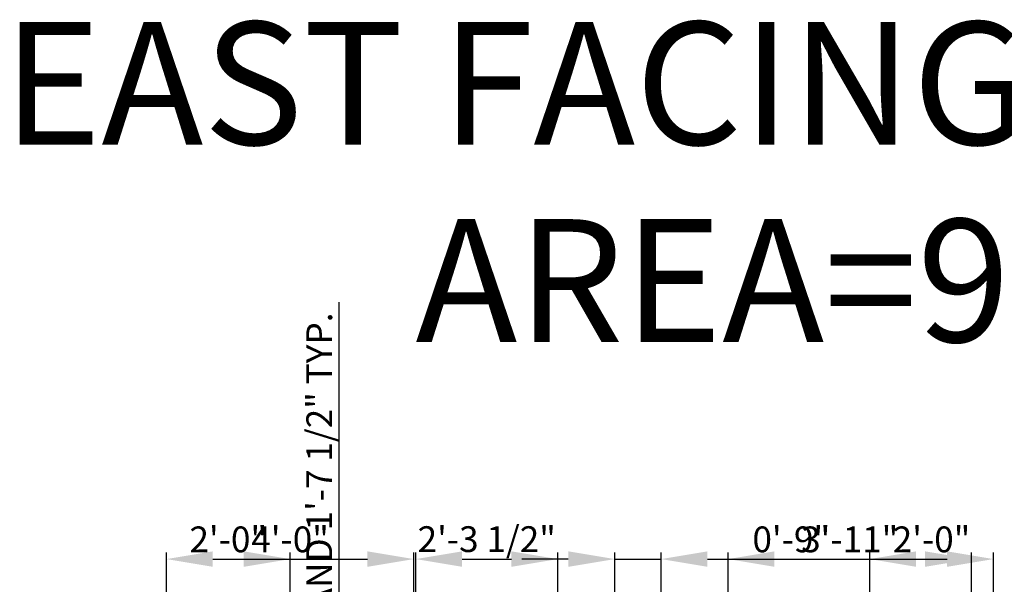
# Model space of a CAD drawing. Units: inches. Extents: x 2265 to 2807, y 1544 to 2401.
# Tile 6 of 9: x 2340 to 2531, y 2291 to 2401. Entities that reach past the tile are written whole.
import ezdxf

# ---------------------------------------------------------------- set-up
doc = ezdxf.new("R2010")
doc.units = ezdxf.units.IN
doc.layers.add('A-ANNO-DIMS', color=2, linetype='Continuous', lineweight=18)
doc.layers.add('A-ANNO-TITL', color=7, linetype='Continuous', lineweight=35)
doc.styles.get("Standard").update_dxf_attribs({"font": 'arial.ttf', "height": 5})
doc.dimstyles.new('ISO-25', dxfattribs={"dimtxt": 5, "dimasz": 9, "dimexe": 1.25, "dimexo": 0.625, "dimtad": 1, "dimlunit": 3, "dimtxsty": 'Standard', "dimcen": 2.5, "dimadec": 0, "dimazin": 0, "dimtfac": 1, "dimtmove": 0, "dimatfit": 3, "dimfxl": 1, "dimarcsym": 0})

# ---------------------------------------------------------------- blocks, each defined once
blk = doc.blocks.new('*D31')
at = {"layer": 'A-ANNO-DIMS', "color": 0, "lineweight": -2, "transparency": 16777216}
for p, q in [((2401.62, 2246.73), (2401.62, 2346.21)), ((2399.29, 2246.73), (2402.87, 2246.73)), ((2401.62, 2236.05), (2401.62, 2237.73)), ((2399.29, 2227.05), (2402.87, 2227.05))]:
    blk.add_line(p, q, dxfattribs=at)
at = {"layer": 'A-ANNO-DIMS', "color": 0, "lineweight": 100, "transparency": 16777216}
for points in [[(2400.12, 2237.73), (2403.12, 2237.73), (2401.62, 2246.73)], [(2400.12, 2236.05), (2403.12, 2236.05), (2401.62, 2227.05)]]:
    blk.add_solid(points, dxfattribs=at)
at = {"layer": 'Defpoints', "color": 0, "lineweight": 100, "transparency": 16777216}
for p in [(2398.67, 2246.73), (2401.62, 2246.73), (2398.67, 2227.05)]:
    blk.add_point(p, dxfattribs=at)
at = {"layer": 'A-ANNO-DIMS', "color": 0, "transparency": 16777216, "insert": (2398.41, 2300.97), "char_height": 5, "attachment_point": 5, "rotation": 90}
blk.add_mtext('NIGHTSTAND 1\'-7 1/2" TYP.', dxfattribs=at)
blk = doc.blocks.new('*D40')
at = {"layer": 'A-ANNO-DIMS', "color": 0, "lineweight": -2, "transparency": 16777216}
for p, q in [((2368.1, 2005.86), (2368.1, 2297.59)), ((2392.1, 2005.86), (2392.1, 2297.59)), ((2377.1, 2296.34), (2383.1, 2296.34))]:
    blk.add_line(p, q, dxfattribs=at)
at = {"layer": 'A-ANNO-DIMS', "color": 0, "lineweight": 100, "transparency": 16777216}
for points in [[(2377.1, 2297.84), (2377.1, 2294.84), (2368.1, 2296.34)], [(2383.1, 2297.84), (2383.1, 2294.84), (2392.1, 2296.34)]]:
    blk.add_solid(points, dxfattribs=at)
at = {"layer": 'Defpoints', "color": 0, "lineweight": 100, "transparency": 16777216}
for p in [(2392.1, 2296.34), (2368.1, 2005.23), (2392.1, 2005.23)]:
    blk.add_point(p, dxfattribs=at)
at = {"layer": 'A-ANNO-DIMS', "color": 0, "transparency": 16777216, "insert": (2380.1, 2299.52), "char_height": 5, "attachment_point": 5}
blk.add_mtext('2\'-0"', dxfattribs=at)
blk = doc.blocks.new('*D43')
at = {"layer": 'A-ANNO-DIMS', "color": 0, "lineweight": -2, "transparency": 16777216}
for p, q in [((2416.49, 1959.08), (2416.49, 2297.59)), ((2444.05, 1959.08), (2444.05, 2297.59)), ((2425.49, 2296.34), (2435.05, 2296.34))]:
    blk.add_line(p, q, dxfattribs=at)
at = {"layer": 'A-ANNO-DIMS', "color": 0, "lineweight": 100, "transparency": 16777216}
for points in [[(2425.49, 2297.84), (2425.49, 2294.84), (2416.49, 2296.34)], [(2435.05, 2297.84), (2435.05, 2294.84), (2444.05, 2296.34)]]:
    blk.add_solid(points, dxfattribs=at)
at = {"layer": 'Defpoints', "color": 0, "lineweight": 100, "transparency": 16777216}
for p in [(2444.05, 2296.34), (2416.49, 1958.45), (2444.05, 1958.45)]:
    blk.add_point(p, dxfattribs=at)
at = {"layer": 'A-ANNO-DIMS', "color": 0, "transparency": 16777216, "insert": (2430.27, 2299.56), "char_height": 5, "attachment_point": 5}
blk.add_mtext('2\'-3 1/2"', dxfattribs=at)
blk = doc.blocks.new('*D47')
at = {"layer": 'A-ANNO-DIMS', "color": 0, "lineweight": -2, "transparency": 16777216}
for p, q in [((2455.1, 2124.36), (2455.1, 2297.59)), ((2464.1, 2124.36), (2464.1, 2297.59)), ((2446.1, 2296.34), (2437.1, 2296.34)), ((2455.1, 2296.34), (2464.1, 2296.34)), ((2473.1, 2296.34), (2496.64, 2296.34))]:
    blk.add_line(p, q, dxfattribs=at)
at = {"layer": 'A-ANNO-DIMS', "color": 0, "lineweight": 100, "transparency": 16777216}
for points in [[(2446.1, 2297.84), (2446.1, 2294.84), (2455.1, 2296.34)], [(2473.1, 2297.84), (2473.1, 2294.84), (2464.1, 2296.34)]]:
    blk.add_solid(points, dxfattribs=at)
at = {"layer": 'Defpoints', "color": 0, "lineweight": 100, "transparency": 16777216}
for p in [(2464.1, 2296.34), (2455.1, 2123.73), (2464.1, 2123.73)]:
    blk.add_point(p, dxfattribs=at)
at = {"layer": 'A-ANNO-DIMS', "color": 0, "transparency": 16777216, "insert": (2489.37, 2299.52), "char_height": 5, "attachment_point": 5}
blk.add_mtext('0\'-9"', dxfattribs=at)
blk = doc.blocks.new('*D54')
at = {"layer": 'A-ANNO-DIMS', "color": 0, "lineweight": -2, "transparency": 16777216}
for p, q in [((2368.1, 2247.36), (2368.1, 2297.59)), ((2416.1, 2247.36), (2416.1, 2297.59)), ((2377.1, 2296.34), (2407.1, 2296.34))]:
    blk.add_line(p, q, dxfattribs=at)
at = {"layer": 'A-ANNO-DIMS', "color": 0, "lineweight": 100, "transparency": 16777216}
for points in [[(2377.1, 2297.84), (2377.1, 2294.84), (2368.1, 2296.34)], [(2407.1, 2297.84), (2407.1, 2294.84), (2416.1, 2296.34)]]:
    blk.add_solid(points, dxfattribs=at)
at = {"layer": 'Defpoints', "color": 0, "lineweight": 100, "transparency": 16777216}
for p in [(2416.1, 2296.34), (2368.1, 2246.73), (2416.1, 2246.73)]:
    blk.add_point(p, dxfattribs=at)
at = {"layer": 'A-ANNO-DIMS', "color": 0, "transparency": 16777216, "insert": (2392.1, 2299.52), "char_height": 5, "attachment_point": 5}
blk.add_mtext('4\'-0"', dxfattribs=at)
blk = doc.blocks.new('*D55')
at = {"layer": 'A-ANNO-DIMS', "color": 0, "lineweight": -2, "transparency": 16777216}
for p, q in [((2504.6, 2247.36), (2504.6, 2297.59)), ((2528.6, 2247.36), (2528.6, 2297.59)), ((2513.6, 2296.34), (2519.6, 2296.34))]:
    blk.add_line(p, q, dxfattribs=at)
at = {"layer": 'A-ANNO-DIMS', "color": 0, "lineweight": 100, "transparency": 16777216}
for points in [[(2513.6, 2297.84), (2513.6, 2294.84), (2504.6, 2296.34)], [(2519.6, 2297.84), (2519.6, 2294.84), (2528.6, 2296.34)]]:
    blk.add_solid(points, dxfattribs=at)
at = {"layer": 'Defpoints', "color": 0, "lineweight": 100, "transparency": 16777216}
for p in [(2528.6, 2296.34), (2504.6, 2246.73), (2528.6, 2246.73)]:
    blk.add_point(p, dxfattribs=at)
at = {"layer": 'A-ANNO-DIMS', "color": 0, "transparency": 16777216, "insert": (2516.6, 2299.52), "char_height": 5, "attachment_point": 5}
blk.add_mtext('2\'-0"', dxfattribs=at)
blk = doc.blocks.new('*D63')
at = {"layer": 'A-ANNO-DIMS', "color": 0, "lineweight": -2, "transparency": 16777216}
for p, q in [((2477.1, 1993.66), (2477.1, 2297.59)), ((2524.34, 1993.66), (2524.34, 2297.59)), ((2486.1, 2296.34), (2515.34, 2296.34))]:
    blk.add_line(p, q, dxfattribs=at)
at = {"layer": 'A-ANNO-DIMS', "color": 0, "lineweight": 100, "transparency": 16777216}
for points in [[(2486.1, 2297.84), (2486.1, 2294.84), (2477.1, 2296.34)], [(2515.34, 2297.84), (2515.34, 2294.84), (2524.34, 2296.34)]]:
    blk.add_solid(points, dxfattribs=at)
at = {"layer": 'Defpoints', "color": 0, "lineweight": 100, "transparency": 16777216}
for p in [(2524.34, 2296.34), (2477.1, 1993.03), (2524.34, 1993.03)]:
    blk.add_point(p, dxfattribs=at)
at = {"layer": 'A-ANNO-DIMS', "color": 0, "transparency": 16777216, "insert": (2500.72, 2299.52), "char_height": 5, "attachment_point": 5}
blk.add_mtext('3\'-11"', dxfattribs=at)

msp = doc.modelspace()

# ---------------------------------------------------------------- texts
at = {"layer": 'A-ANNO-TITL'}
for s, p in [('EAST FACING  HOUSE', (2336.336, 2376.748)), ('           AREA=975sq.ft', (2336.336, 2338.469))]:
    msp.add_text(s, height=23.82874, dxfattribs=at).set_placement(p)

# ---------------------------------------------------------------- dimensions: what is measured, and where the dimension line sits
at = {"layer": 'A-ANNO-DIMS'}
dim = msp.add_linear_dim(base=(2401.621, 2246.733), p1=(2398.668, 2227.048), p2=(2398.668, 2246.733), angle=90, text='NIGHTSTAND <> TYP.', dimstyle='ISO-25', override={"dimdec": 1, "dimlfac": 1, "dimrnd": 0, "dimzin": 1, "dimdsep": 46, "dimlunit": 4, "dimfrac": 2}, dxfattribs=at)
dim.commit()
dim.dimension.update_dxf_attribs({"geometry": '*D31', "text_midpoint": (2398.411, 2300.973)})
for base, p1, p2, picture, middle in [((2444.049, 2296.343), (2416.49, 1958.452), (2444.049, 1958.452), '*D43', (2430.27, 2299.555)), ((2392.101, 2296.343), (2368.101, 2005.233), (2392.101, 2005.233), '*D40', (2380.101, 2299.521)), ((2416.101, 2296.343), (2368.101, 2246.733), (2416.101, 2246.733), '*D54', (2392.101, 2299.521)), ((2464.101, 2296.343), (2455.101, 2123.733), (2464.101, 2123.733), '*D47', (2489.372, 2299.521)), ((2524.342, 2296.343), (2477.098, 1993.031), (2524.342, 1993.031), '*D63', (2500.72, 2299.523)), ((2528.601, 2296.343), (2504.601, 2246.733), (2528.601, 2246.733), '*D55', (2516.601, 2299.521))]:
    dim = msp.add_linear_dim(base=base, p1=p1, p2=p2, dimstyle='ISO-25', override={"dimdec": 1, "dimlfac": 1, "dimrnd": 0, "dimzin": 1, "dimdsep": 46, "dimlunit": 4, "dimfrac": 2}, dxfattribs=at)
    dim.commit()
    dim.dimension.update_dxf_attribs({"geometry": picture, "text_midpoint": middle})

doc.saveas('drawing.dxf')
